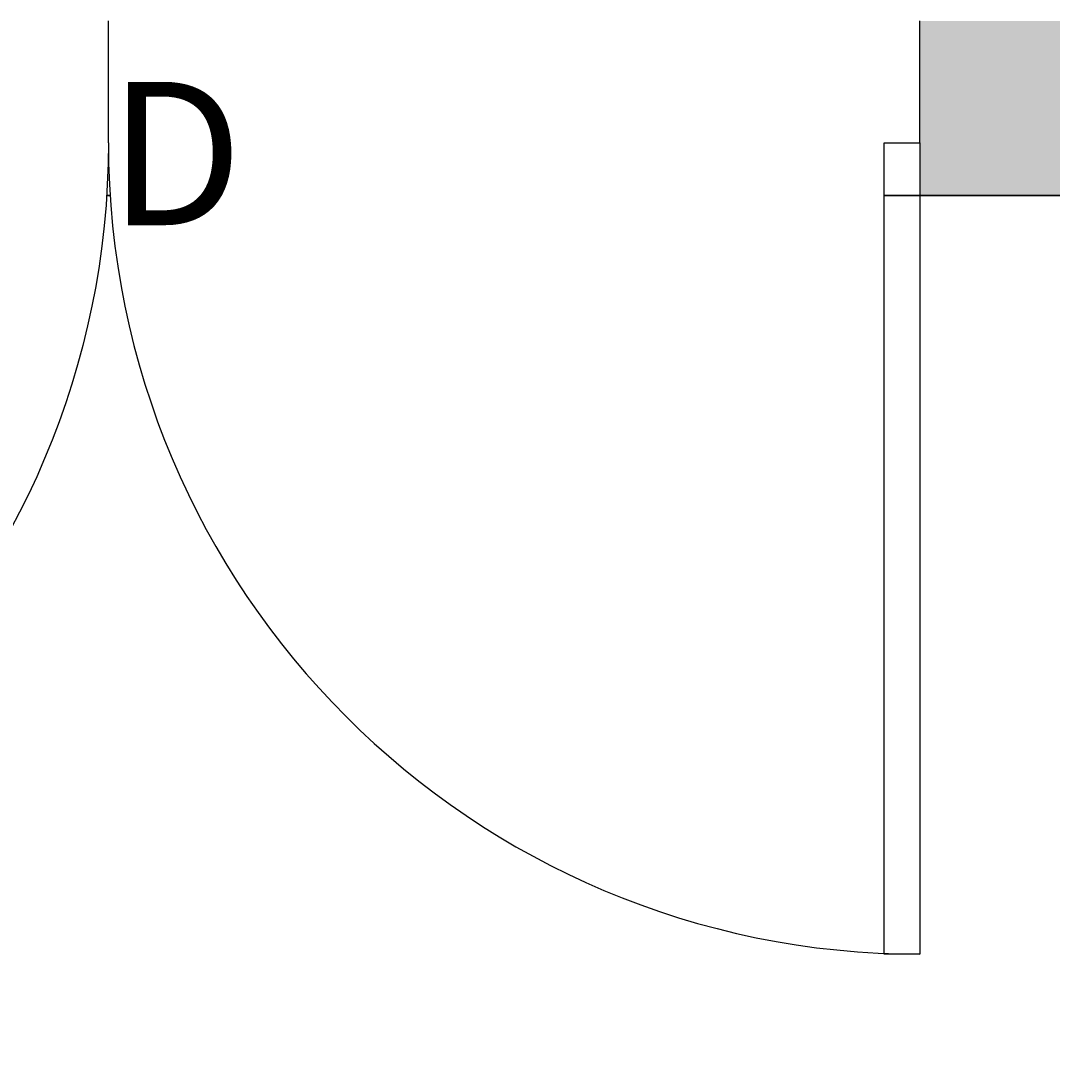
# Model space of a CAD drawing. Units: inches. Extents: x 1998 to 2588, y 1139 to 1977.
# Tile 79 of 134: x 2370 to 2397, y 1454 to 1481. Entities that reach past the tile are written whole.
import ezdxf

# ---------------------------------------------------------------- set-up
doc = ezdxf.new("R2010")
doc.units = ezdxf.units.IN
for name, color, linetype, lineweight in [('A-ANNO-DIMS', 2, 'Continuous', 18), ('A-DOOR-IDEN', 7, 'Continuous', 18), ('A-WALL-PATT', 252, 'Continuous', 13), ('DOOR', 52, 'Continuous', 25), ('WALL', 200, 'Continuous', 35)]:
    doc.layers.add(name, color=color, linetype=linetype, lineweight=lineweight)
doc.styles.get("Standard").update_dxf_attribs({"font": 'arial.ttf'})
doc.dimstyles.get("Standard").update_dxf_attribs({"dimtxt": 0.18, "dimasz": 0.18, "dimexe": 0.18, "dimexo": 0.0625, "dimgap": 0.09, "dimtad": 0, "dimtih": 1, "dimtoh": 1, "dimdec": 4, "dimzin": 0, "dimdsep": 46, "dimtxsty": 'Standard', "dimcen": 0.09, "dimadec": 0, "dimazin": 0, "dimtfac": 1, "dimtdec": 4, "dimtofl": 0, "dimtmove": 0, "dimatfit": 3, "dimfxl": 1, "dimtolj": 1, "dimtzin": 0, "dimarcsym": 0})

# ---------------------------------------------------------------- blocks, each defined once
blk = doc.blocks.new('*U2')
for p, q in [((0, 0), (0, -6)), ((40, 0), (40, -6))]:
    blk.add_line(p, q)
blk.add_lwpolyline([(0, 0), (0, 40), (1.75, 40), (1.75, 0)], close=True)
blk.add_arc((0, 0), 40, 0, 90)
blk = doc.blocks.new('*D23')
at = {"layer": 'A-ANNO-DIMS', "color": 0, "lineweight": -2, "transparency": 16777216}
for p, q in [((2549.179, 1476.17), (2549.179, 1138.602)), ((2059.473, 1413.17), (2059.473, 1138.602)), ((2059.653, 1138.782), (2303.928, 1138.782)), ((2548.999, 1138.782), (2304.723, 1138.782))]:
    blk.add_line(p, q, dxfattribs=at)
at = {"layer": 'A-ANNO-DIMS', "color": 0, "transparency": 16777216}
for points in [[(2059.653, 1138.812), (2059.653, 1138.752), (2059.473, 1138.782)], [(2548.999, 1138.812), (2548.999, 1138.752), (2549.179, 1138.782)]]:
    blk.add_solid(points, dxfattribs=at)
at = {"layer": 'Defpoints', "color": 0, "transparency": 16777216}
for p in [(2549.179, 1476.232), (2059.473, 1413.232), (2549.179, 1138.782)]:
    blk.add_point(p, dxfattribs=at)
at = {"layer": 'A-ANNO-DIMS', "color": 0, "transparency": 16777216, "insert": (2304.326, 1138.782), "char_height": 0.18, "attachment_point": 5}
blk.add_mtext('\\A1;489.7', dxfattribs=at)
blk = doc.blocks.new('*D43')
at = {"layer": 'A-ANNO-DIMS', "color": 0, "lineweight": -2, "transparency": 16777216}
for p, q in [((2407.973, 1594.67), (2407.973, 1138.602)), ((2345.973, 1588.67), (2345.973, 1138.602)), ((2346.153, 1138.782), (2376.754, 1138.782)), ((2407.793, 1138.782), (2377.191, 1138.782))]:
    blk.add_line(p, q, dxfattribs=at)
at = {"layer": 'A-ANNO-DIMS', "color": 0, "transparency": 16777216}
for points in [[(2346.153, 1138.812), (2346.153, 1138.752), (2345.973, 1138.782)], [(2407.793, 1138.812), (2407.793, 1138.752), (2407.973, 1138.782)]]:
    blk.add_solid(points, dxfattribs=at)
at = {"layer": 'Defpoints', "color": 0, "transparency": 16777216}
for p in [(2407.973, 1594.732), (2345.973, 1588.732), (2407.973, 1138.782)]:
    blk.add_point(p, dxfattribs=at)
at = {"layer": 'A-ANNO-DIMS', "color": 0, "transparency": 16777216, "insert": (2376.973, 1138.782), "char_height": 0.18, "attachment_point": 5}
blk.add_mtext('\\A1;62', dxfattribs=at)

msp = doc.modelspace()

# ---------------------------------------------------------------- hatches: boundary and pattern name
at = {"layer": 'A-WALL-PATT'}
h = msp.add_hatch(color=256, dxfattribs=at)
h.dxf.hatch_style = 1
h.paths.add_polyline_path([(2527.4729, 1362.2324), (2510.9729, 1362.2324), (2510.9729, 1357.7324), (2518.4729, 1357.7324), (2518.4729, 1237.7324), (2503.1458, 1237.7324), (2503.1458, 1228.7324), (2527.4729, 1228.7324)])
h.paths.add_polyline_path([(2490.5682, 1362.2324), (2398.4729, 1362.2324), (2398.4729, 1357.7324), (2490.5682, 1357.7324)])
h.paths.add_polyline_path([(2224.9729, 1264.7324), (2222.9729, 1264.7324), (2222.9729, 1232.4125), (2341.4729, 1232.4125), (2341.4729, 1234.4125), (2224.9729, 1234.4125)])
h.paths.add_polyline_path([(2334.5332, 1273.7324), (2264.7638, 1273.7324), (2264.7638, 1269.5611, -0.043659), (2264.3413, 1264.7324), (2334.5332, 1264.7324)])
h.paths.add_polyline_path([(2236.9551, 1273.7324), (2234.4125, 1273.7324), (2234.4125, 1264.7324), (2236.9551, 1264.7324), (2236.9551, 1269.5611)])
h.paths.add_polyline_path([(2222.9729, 1293.2324), (2096.9729, 1293.2324), (2096.9729, 1345.0966), (2087.9729, 1345.0966), (2087.9729, 1284.2324), (2222.9729, 1284.2324), (2222.9729, 1285.137)])
h.paths.add_polyline_path([(2096.9729, 1458.7927), (2087.9729, 1458.7927), (2087.9729, 1417.7324), (2087.9729, 1413.2324), (2096.9729, 1413.2324), (2096.9729, 1417.7324)])
h.paths.add_polyline_path([(2096.9729, 1413.2324), (2087.9729, 1413.2324), (2087.9729, 1365.5012), (2096.9729, 1365.5012), (2096.9729, 1369.3358)])
h.paths.add_polyline_path([(2186.2943, 1417.7324), (2138.6074, 1417.7324), (2096.9729, 1417.7324), (2096.9729, 1413.2324), (2138.6074, 1413.2324), (2186.2943, 1413.2324)])
h.paths.add_polyline_path([(2181.4729, 1465.7324), (2176.9729, 1465.7324), (2176.9729, 1451.6434), (2181.4729, 1451.6434)])
h.paths.add_polyline_path([(2181.4729, 1422.1664), (2176.9729, 1422.1664), (2176.9729, 1417.7324), (2181.4729, 1417.7324)])
h.paths.add_polyline_path([(2063.9729, 1465.7324), (2087.9729, 1465.7324), (2087.9729, 1470.2324), (2059.4729, 1470.2324), (2059.4729, 1413.2324), (2087.9729, 1413.2324), (2087.9729, 1417.7324), (2063.9729, 1417.7324)])
h.paths.add_polyline_path([(2181.4729, 1755.2324), (2176.9729, 1755.2324), (2176.9729, 1748.6798), (2177.0513, 1748.6798), (2181.4729, 1748.6798)])
h.paths.add_polyline_path([(2227.4729, 1707.2324), (2220.4647, 1707.2324), (2220.4647, 1702.7324), (2222.9729, 1702.7324), (2222.9729, 1604.637), (2227.4729, 1604.637)])
h.paths.add_polyline_path([(2114.9729, 1702.7324), (2105.9729, 1702.7324), (2105.9729, 1628.4781, -0.0318759), (2110.1012, 1628.7416), (2114.9729, 1628.7416)])
h.paths.add_polyline_path([(2345.9729, 1739.3278), (2341.4729, 1739.3278), (2341.4729, 1647.5211), (2345.9729, 1647.5211)])
h.paths.add_polyline_path([(2350.6273, 1641.2324), (2345.9729, 1641.2324), (2345.9729, 1636.7324), (2350.6273, 1636.7324), (2350.6273, 1639.8729)])
h.paths.add_polyline_path([(2501.9729, 1641.2324), (2407.9729, 1641.2324), (2392.5005, 1641.2324), (2392.5005, 1639.8729), (2392.5005, 1636.7324), (2501.9729, 1636.7324)])
h.paths.add_polyline_path([(2510.9729, 1755.2324), (2501.9729, 1755.2324), (2501.9729, 1641.2324), (2510.9729, 1641.2324)])
h.paths.add_polyline_path([(2549.1786, 1641.2324), (2522.3775, 1641.2324), (2522.3775, 1636.7324), (2540.1786, 1636.7324), (2540.1786, 1480.7324), (2522.3775, 1480.7324), (2522.3775, 1476.2324), (2549.1786, 1476.2324)])
h.paths.add_polyline_path([(2498.1786, 1594.7324), (2407.9729, 1594.7324), (2407.9729, 1585.7324), (2416.9729, 1585.7324), (2489.1786, 1585.7324), (2489.1786, 1531.7324), (2416.9729, 1531.7324), (2407.9729, 1531.7324), (2407.9729, 1522.7324), (2498.1786, 1522.7324)])
h.paths.add_polyline_path([(2351.6437, 1480.7324), (2345.9729, 1480.7324), (2345.9729, 1476.2324), (2351.6437, 1476.2324), (2351.6437, 1477.5919)])
h.paths.add_polyline_path([(2501.9729, 1480.7324), (2498.1786, 1480.7324), (2407.9729, 1480.7324), (2393.5168, 1480.7324), (2393.5168, 1477.5919), (2393.5168, 1476.2324), (2501.9729, 1476.2324)])

# ---------------------------------------------------------------- linework, layer by layer
at = {"layer": 'WALL'}
for p, q in [((2372.536, 1476.2324), (2372.6244, 1476.2324)), ((2372.536, 1476.2324), (2372.6244, 1476.2324)), ((2392.6008, 1476.2324), (2407.9729, 1476.2324)), ((2392.6008, 1476.2324), (2501.9729, 1476.2324))]:
    msp.add_line(p, q, dxfattribs=at)

# ---------------------------------------------------------------- block references
at = {"layer": 'DOOR', "yscale": 0.5234138920659225, "zscale": 0.5234138920659225, "rotation": 180}
for p, xscale in [((2351.6437, 1477.5919), -0.5234138920659225), ((2393.5168, 1477.5919), 0.5234138920659225)]:
    msp.add_blockref('*U2', p, dxfattribs=dict(at, xscale=xscale))

# ---------------------------------------------------------------- texts
at = {"layer": 'A-DOOR-IDEN', "insert": (2372.5802, 1479.1621), "char_height": 3.6988, "attachment_point": 1}
msp.add_mtext_dynamic_manual_height_columns('D', width=110.572713, gutter_width=18.4938, heights=[0], dxfattribs=at)

# ---------------------------------------------------------------- dimensions: what is measured, and where the dimension line sits
at = {"layer": 'A-ANNO-DIMS'}
for base, p1, p2, override, picture, middle in [((2407.9729, 1138.7824), (2345.9729, 1588.7324), (2407.9729, 1594.7324), {"dimdec": 0, "dimlfac": 1, "dimrnd": 0, "dimzin": 0, "dimdsep": 46, "dimlunit": 2}, '*D43', (2376.9729, 1138.7824)), ((2549.1786, 1138.7824), (2059.4729, 1413.2324), (2549.1786, 1476.2324), {"dimdec": 1, "dimlfac": 1, "dimrnd": 0, "dimzin": 0, "dimdsep": 46, "dimlunit": 2}, '*D23', (2304.3257, 1138.7824))]:
    dim = msp.add_linear_dim(base=base, p1=p1, p2=p2, dimstyle='Standard', override=override, dxfattribs=at)
    dim.commit()
    dim.dimension.update_dxf_attribs({"geometry": picture, "text_midpoint": middle})

doc.saveas('drawing.dxf')
